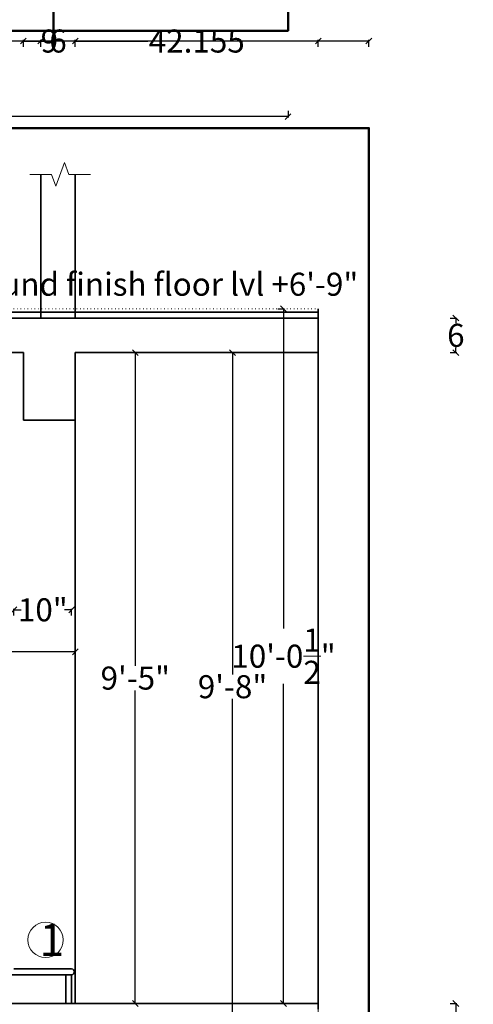
# Model space of a CAD drawing. Units: inches. Extents: x -60 to 284, y -245 to 257.
# Tile 5 of 10: x 193 to 272, y -159 to 12. Entities that reach past the tile are written whole.
import ezdxf

# ---------------------------------------------------------------- set-up
doc = ezdxf.new("R2010")
doc.units = ezdxf.units.IN
doc.header["$LTSCALE"] = 0.8
doc.header["$MEASUREMENT"] = 0
doc.linetypes.add('DOT', pattern=[6.35, 0, -6.35])
for name, color, linetype, lineweight in [('A-ANNO-DIMS', 2, 'Continuous', 18), ('A-ANNO-SYMB', 3, 'Continuous', 18), ('A-ANNO-TEXT', 3, 'Continuous', 18), ('A-ANNO-TTLB', 7, 'Continuous', 50), ('A-SECT', 7, 'Continuous', 35), ('A-SECT-OVHD', 8, 'DOT', 18), ('A-WALL', 7, 'Continuous', 50)]:
    doc.layers.add(name, color=color, linetype=linetype, lineweight=lineweight)
doc.styles.get("Standard").update_dxf_attribs({"font": 'arial.ttf'})
doc.dimstyles.get("Standard").update_dxf_attribs({"dimtxt": 4, "dimasz": 1, "dimexe": 0.18, "dimexo": 0.0625, "dimgap": 0.09, "dimtad": 0, "dimtih": 1, "dimtoh": 1, "dimzin": 0, "dimdsep": 46, "dimlunit": 4, "dimtxsty": 'Standard', "dimblk": 'OBLIQUE', "dimcen": 0.09, "dimadec": 0, "dimazin": 0, "dimtfac": 1, "dimtofl": 0, "dimtmove": 0, "dimatfit": 3, "dimfxl": 1, "dimfxlon": 1, "dimtolj": 1, "dimtzin": 0, "dimarcsym": 0})

# ---------------------------------------------------------------- blocks, each defined once
blk = doc.blocks.new('_Oblique')
at = {"color": 0, "linetype": 'ByBlock', "lineweight": -2}
blk.add_line((-0.5, -0.5), (0.5, 0.5), dxfattribs=at)
blk = doc.blocks.new('*D41')
at = {"layer": 'A-ANNO-DIMS', "color": 0, "lineweight": -2, "ltscale": 0.8, "transparency": 16777216}
for p, q in [((192.1, -91.86), (192.1, -90.68)), ((192.1, -90.86), (193.35, -90.86)), ((202.1, -90.86), (200.85, -90.86)), ((202.1, -91.86), (202.1, -90.68))]:
    blk.add_line(p, q, dxfattribs=at)
at = {"layer": 'Defpoints', "color": 0, "ltscale": 0.8, "transparency": 16777216}
for p in [(192.1, -90.86), (192.1, -168.75), (202.1, -168.75)]:
    blk.add_point(p, dxfattribs=at)
at = {"layer": 'A-ANNO-DIMS', "color": 0, "lineweight": -2, "ltscale": 0.8, "transparency": 16777216, "rotation": 180}
blk.add_blockref('_Oblique', (192.1, -90.86), dxfattribs=at)
at = {"layer": 'A-ANNO-DIMS', "color": 0, "lineweight": -2, "ltscale": 0.8, "transparency": 16777216}
blk.add_blockref('_Oblique', (202.1, -90.86), dxfattribs=at)
at = {"layer": 'A-ANNO-DIMS', "color": 0, "ltscale": 0.8, "transparency": 16777216, "insert": (197.1, -90.86), "char_height": 4, "attachment_point": 5}
blk.add_mtext('\\A1;10"', dxfattribs=at)
blk = doc.blocks.new('*D68')
at = {"layer": 'A-ANNO-DIMS', "color": 0, "lineweight": -2, "ltscale": 0.8, "transparency": 16777216}
for p, q in [((67.01, -97.15), (67.01, -98.33)), ((202.74, -97.15), (202.74, -98.33)), ((67.01, -98.15), (126.59, -98.15)), ((202.74, -98.15), (143.17, -98.15))]:
    blk.add_line(p, q, dxfattribs=at)
at = {"layer": 'Defpoints', "color": 0, "ltscale": 0.8, "transparency": 16777216}
for p in [(67.01, -93.21), (202.74, -93.21), (202.74, -98.15)]:
    blk.add_point(p, dxfattribs=at)
at = {"layer": 'A-ANNO-DIMS', "color": 0, "lineweight": -2, "ltscale": 0.8, "transparency": 16777216, "rotation": 180}
blk.add_blockref('_Oblique', (67.01, -98.15), dxfattribs=at)
at = {"layer": 'A-ANNO-DIMS', "color": 0, "lineweight": -2, "ltscale": 0.8, "transparency": 16777216}
blk.add_blockref('_Oblique', (202.74, -98.15), dxfattribs=at)
at = {"layer": 'A-ANNO-DIMS', "color": 0, "ltscale": 0.8, "transparency": 16777216, "insert": (134.88, -98.15), "char_height": 4, "attachment_point": 5}
blk.add_mtext('\\A1;11\'-3{\\H1x;\\S3/4;}"', dxfattribs=at)
blk = doc.blocks.new('*D69')
at = {"layer": 'A-ANNO-DIMS', "color": 0, "lineweight": -2, "ltscale": 0.8, "transparency": 16777216}
for p, q in [((212.15, -46.21), (213.33, -46.21)), ((213.15, -46.21), (213.15, -100.58)), ((213.15, -159.21), (213.15, -104.84)), ((212.15, -159.21), (213.33, -159.21))]:
    blk.add_line(p, q, dxfattribs=at)
at = {"layer": 'Defpoints', "color": 0, "ltscale": 0.8, "transparency": 16777216}
for p in [(212.05, -46.21), (213.15, -46.21), (212.05, -159.21)]:
    blk.add_point(p, dxfattribs=at)
at = {"layer": 'A-ANNO-DIMS', "color": 0, "lineweight": -2, "ltscale": 0.8, "transparency": 16777216}
for p, rotation in [((213.15, -46.21), 90), ((213.15, -159.21), 270)]:
    blk.add_blockref('_Oblique', p, dxfattribs=dict(at, rotation=rotation))
at = {"layer": 'A-ANNO-DIMS', "color": 0, "ltscale": 0.8, "transparency": 16777216, "insert": (213.15, -102.71), "char_height": 4, "attachment_point": 5}
blk.add_mtext('\\A1;9\'-5"', dxfattribs=at)
blk = doc.blocks.new('*D70')
at = {"layer": 'A-ANNO-DIMS', "color": 0, "lineweight": -2, "ltscale": 0.8, "transparency": 16777216}
for p, q in [((229.03, -46.21), (230.21, -46.21)), ((230.03, -46.21), (230.03, -102.08)), ((230.03, -162.21), (230.03, -106.34)), ((229.03, -162.21), (230.21, -162.21))]:
    blk.add_line(p, q, dxfattribs=at)
at = {"layer": 'Defpoints', "color": 0, "ltscale": 0.8, "transparency": 16777216}
for p in [(227.81, -46.21), (230.03, -46.21), (219.24, -162.21)]:
    blk.add_point(p, dxfattribs=at)
at = {"layer": 'A-ANNO-DIMS', "color": 0, "lineweight": -2, "ltscale": 0.8, "transparency": 16777216}
for p, rotation in [((230.03, -46.21), 90), ((230.03, -162.21), 270)]:
    blk.add_blockref('_Oblique', p, dxfattribs=dict(at, rotation=rotation))
at = {"layer": 'A-ANNO-DIMS', "color": 0, "ltscale": 0.8, "transparency": 16777216, "insert": (230.03, -104.21), "char_height": 4, "attachment_point": 5}
blk.add_mtext('\\A1;9\'-8"', dxfattribs=at)
blk = doc.blocks.new('*D71')
at = {"layer": 'A-ANNO-DIMS', "color": 0, "lineweight": -2, "ltscale": 0.8, "transparency": 16777216}
for p, q in [((237.88, -38.61), (239.06, -38.61)), ((238.88, -38.61), (238.88, -94.1)), ((238.88, -159.21), (238.88, -103.72)), ((237.88, -159.21), (239.06, -159.21))]:
    blk.add_line(p, q, dxfattribs=at)
at = {"layer": 'Defpoints', "color": 0, "ltscale": 0.8, "transparency": 16777216}
for p in [(235.46, -38.61), (238.88, -38.61), (235.46, -159.21)]:
    blk.add_point(p, dxfattribs=at)
at = {"layer": 'A-ANNO-DIMS', "color": 0, "lineweight": -2, "ltscale": 0.8, "transparency": 16777216}
for p, rotation in [((238.88, -38.61), 90), ((238.88, -159.21), 270)]:
    blk.add_blockref('_Oblique', p, dxfattribs=dict(at, rotation=rotation))
at = {"layer": 'A-ANNO-DIMS', "color": 0, "ltscale": 0.8, "transparency": 16777216, "insert": (238.88, -98.91), "char_height": 4, "attachment_point": 5}
blk.add_mtext('\\A1;10\'-0{\\H1x;\\S1/2;}"', dxfattribs=at)
blk = doc.blocks.new('*D89')
at = {"layer": 'A-ANNO-DIMS', "color": 0, "lineweight": -2, "ltscale": 0.8, "transparency": 16777216}
for p, q in [((0.09, -4.23), (0.09, -5.41)), ((239.66, -4.23), (239.66, -5.41)), ((0.09, -5.23), (113, -5.23)), ((239.66, -5.23), (126.75, -5.23))]:
    blk.add_line(p, q, dxfattribs=at)
at = {"layer": 'Defpoints', "color": 0, "ltscale": 0.8, "transparency": 16777216}
for p in [(0.09, 9.67), (239.66, 9.67), (239.66, -5.23)]:
    blk.add_point(p, dxfattribs=at)
at = {"layer": 'A-ANNO-DIMS', "color": 0, "lineweight": -2, "ltscale": 0.8, "transparency": 16777216, "rotation": 180}
blk.add_blockref('_Oblique', (0.09, -5.23), dxfattribs=at)
at = {"layer": 'A-ANNO-DIMS', "color": 0, "lineweight": -2, "ltscale": 0.8, "transparency": 16777216}
blk.add_blockref('_Oblique', (239.66, -5.23), dxfattribs=at)
at = {"layer": 'A-ANNO-DIMS', "color": 0, "ltscale": 0.8, "transparency": 16777216, "insert": (119.88, -5.23), "char_height": 4, "attachment_point": 5}
blk.add_mtext('\\A1;239.6', dxfattribs=at)
blk = doc.blocks.new('*D105')
at = {"layer": 'A-ANNO-DIMS', "color": 0, "lineweight": -2, "ltscale": 0.8, "transparency": 16777216}
for p, q in [((67.01, -241.38), (67.01, -242.56)), ((67.01, -242.38), (149.3, -242.38)), ((244.9, -242.38), (162.61, -242.38)), ((244.9, -241.38), (244.9, -242.56))]:
    blk.add_line(p, q, dxfattribs=at)
at = {"layer": 'Defpoints', "color": 0, "ltscale": 0.8, "transparency": 16777216}
for p in [(67.01, -159.21), (244.9, -171.21), (244.9, -242.38)]:
    blk.add_point(p, dxfattribs=at)
at = {"layer": 'A-ANNO-DIMS', "color": 0, "lineweight": -2, "ltscale": 0.8, "transparency": 16777216, "rotation": 180}
blk.add_blockref('_Oblique', (67.01, -242.38), dxfattribs=at)
at = {"layer": 'A-ANNO-DIMS', "color": 0, "lineweight": -2, "ltscale": 0.8, "transparency": 16777216}
blk.add_blockref('_Oblique', (244.9, -242.38), dxfattribs=at)
at = {"layer": 'A-ANNO-DIMS', "color": 0, "ltscale": 0.8, "transparency": 16777216, "insert": (155.96, -242.38), "char_height": 4, "attachment_point": 5}
blk.add_mtext('\\A1;177.9', dxfattribs=at)
blk = doc.blocks.new('*D107')
at = {"layer": 'A-ANNO-DIMS', "color": 0, "lineweight": -2, "ltscale": 0.8, "transparency": 16777216}
for p, q in [((267.79, -40.21), (268.97, -40.21)), ((268.79, -40.21), (268.79, -41.08)), ((268.79, -46.21), (268.79, -45.34)), ((267.79, -46.21), (268.97, -46.21))]:
    blk.add_line(p, q, dxfattribs=at)
at = {"layer": 'Defpoints', "color": 0, "ltscale": 0.8, "transparency": 16777216}
for p in [(244.9, -40.21), (244.9, -46.21), (268.79, -46.21)]:
    blk.add_point(p, dxfattribs=at)
at = {"layer": 'A-ANNO-DIMS', "color": 0, "lineweight": -2, "ltscale": 0.8, "transparency": 16777216}
for p, rotation in [((268.79, -40.21), 90), ((268.79, -46.21), 270)]:
    blk.add_blockref('_Oblique', p, dxfattribs=dict(at, rotation=rotation))
at = {"layer": 'A-ANNO-DIMS', "color": 0, "ltscale": 0.8, "transparency": 16777216, "insert": (268.79, -43.21), "char_height": 4, "attachment_point": 5}
blk.add_mtext('\\A1;6', dxfattribs=at)
blk = doc.blocks.new('*D108')
at = {"layer": 'A-ANNO-DIMS', "color": 0, "lineweight": -2, "ltscale": 0.8, "transparency": 16777216}
for p, q in [((267.79, -159.21), (268.97, -159.21)), ((268.79, -159.21), (268.79, -163.11)), ((268.79, -171.21), (268.79, -167.31)), ((267.79, -171.21), (268.97, -171.21))]:
    blk.add_line(p, q, dxfattribs=at)
at = {"layer": 'Defpoints', "color": 0, "ltscale": 0.8, "transparency": 16777216}
for p in [(244.9, -159.21), (244.9, -171.21), (268.79, -171.21)]:
    blk.add_point(p, dxfattribs=at)
at = {"layer": 'A-ANNO-DIMS', "color": 0, "lineweight": -2, "ltscale": 0.8, "transparency": 16777216}
for p, rotation in [((268.79, -159.21), 90), ((268.79, -171.21), 270)]:
    blk.add_blockref('_Oblique', p, dxfattribs=dict(at, rotation=rotation))
at = {"layer": 'A-ANNO-DIMS', "color": 0, "ltscale": 0.8, "transparency": 16777216, "insert": (268.79, -165.21), "char_height": 4, "attachment_point": 5}
blk.add_mtext('\\A1;12', dxfattribs=at)
blk = doc.blocks.new('*D109')
at = {"layer": 'A-ANNO-DIMS', "color": 0, "lineweight": -2, "ltscale": 0.8, "transparency": 16777216}
for p, q in [((196.74, 6.88), (196.74, 8.06)), ((196.74, 7.88), (198.33, 7.88)), ((202.74, 7.88), (201.15, 7.88)), ((202.74, 6.88), (202.74, 8.06))]:
    blk.add_line(p, q, dxfattribs=at)
at = {"layer": 'Defpoints', "color": 0, "ltscale": 0.8, "transparency": 16777216}
for p in [(202.74, 7.88), (196.74, -15.28), (202.74, -15.28)]:
    blk.add_point(p, dxfattribs=at)
at = {"layer": 'A-ANNO-DIMS', "color": 0, "lineweight": -2, "ltscale": 0.8, "transparency": 16777216, "rotation": 180}
blk.add_blockref('_Oblique', (196.74, 7.88), dxfattribs=at)
at = {"layer": 'A-ANNO-DIMS', "color": 0, "lineweight": -2, "ltscale": 0.8, "transparency": 16777216}
blk.add_blockref('_Oblique', (202.74, 7.88), dxfattribs=at)
at = {"layer": 'A-ANNO-DIMS', "color": 0, "ltscale": 0.8, "transparency": 16777216, "insert": (199.74, 7.88), "char_height": 4, "attachment_point": 5}
blk.add_mtext('\\A1;6', dxfattribs=at)
blk = doc.blocks.new('*D110')
at = {"layer": 'A-ANNO-DIMS', "color": 0, "lineweight": -2, "ltscale": 0.8, "transparency": 16777216}
for p, q in [((193.74, 6.88), (193.74, 8.06)), ((193.74, 7.88), (196.84, 7.88)), ((202.74, 7.88), (199.65, 7.88)), ((202.74, 6.88), (202.74, 8.06))]:
    blk.add_line(p, q, dxfattribs=at)
at = {"layer": 'Defpoints', "color": 0, "ltscale": 0.8, "transparency": 16777216}
for p in [(202.74, 7.88), (193.74, -57.93), (202.74, -57.93)]:
    blk.add_point(p, dxfattribs=at)
at = {"layer": 'A-ANNO-DIMS', "color": 0, "lineweight": -2, "ltscale": 0.8, "transparency": 16777216, "rotation": 180}
blk.add_blockref('_Oblique', (193.74, 7.88), dxfattribs=at)
at = {"layer": 'A-ANNO-DIMS', "color": 0, "lineweight": -2, "ltscale": 0.8, "transparency": 16777216}
blk.add_blockref('_Oblique', (202.74, 7.88), dxfattribs=at)
at = {"layer": 'A-ANNO-DIMS', "color": 0, "ltscale": 0.8, "transparency": 16777216, "insert": (198.24, 7.88), "char_height": 4, "attachment_point": 5}
blk.add_mtext('\\A1;9', dxfattribs=at)
blk = doc.blocks.new('*D111')
at = {"layer": 'A-ANNO-DIMS', "color": 0, "lineweight": -2, "ltscale": 0.8, "transparency": 16777216}
for p, q in [((-50.85, -46.21), (-52.03, -46.21)), ((-51.85, -46.21), (-51.85, -49.97)), ((-51.85, -57.93), (-51.85, -54.17)), ((-50.85, -57.93), (-52.03, -57.93))]:
    blk.add_line(p, q, dxfattribs=at)
at = {"layer": 'Defpoints', "color": 0, "ltscale": 0.8, "transparency": 16777216}
for p in [(193.74, -46.21), (-51.85, -57.93), (193.74, -57.93)]:
    blk.add_point(p, dxfattribs=at)
at = {"layer": 'A-ANNO-DIMS', "color": 0, "lineweight": -2, "ltscale": 0.8, "transparency": 16777216}
for p, rotation in [((-51.85, -46.21), 90), ((-51.85, -57.93), 270)]:
    blk.add_blockref('_Oblique', p, dxfattribs=dict(at, rotation=rotation))
at = {"layer": 'A-ANNO-DIMS', "color": 0, "ltscale": 0.8, "transparency": 16777216, "insert": (-51.85, -52.07), "char_height": 4, "attachment_point": 5}
blk.add_mtext('\\A1;11.717', dxfattribs=at)
blk = doc.blocks.new('*D112')
at = {"layer": 'A-ANNO-DIMS', "color": 0, "lineweight": -2, "ltscale": 0.8, "transparency": 16777216}
for p, q in [((202.74, 6.88), (202.74, 8.06)), ((202.74, 7.88), (215.33, 7.88)), ((244.9, 7.88), (232.31, 7.88)), ((244.9, 6.88), (244.9, 8.06))]:
    blk.add_line(p, q, dxfattribs=at)
at = {"layer": 'Defpoints', "color": 0, "ltscale": 0.8, "transparency": 16777216}
for p in [(244.9, 7.88), (202.74, -46.21), (244.9, -46.21)]:
    blk.add_point(p, dxfattribs=at)
at = {"layer": 'A-ANNO-DIMS', "color": 0, "lineweight": -2, "ltscale": 0.8, "transparency": 16777216, "rotation": 180}
blk.add_blockref('_Oblique', (202.74, 7.88), dxfattribs=at)
at = {"layer": 'A-ANNO-DIMS', "color": 0, "lineweight": -2, "ltscale": 0.8, "transparency": 16777216}
blk.add_blockref('_Oblique', (244.9, 7.88), dxfattribs=at)
at = {"layer": 'A-ANNO-DIMS', "color": 0, "ltscale": 0.8, "transparency": 16777216, "insert": (223.82, 7.88), "char_height": 4, "attachment_point": 5}
blk.add_mtext('\\A1;42.155', dxfattribs=at)
blk = doc.blocks.new('*D114')
at = {"layer": 'A-ANNO-DIMS', "color": 0, "lineweight": -2, "ltscale": 0.8, "transparency": 16777216}
for p, q in [((-36.75, 6.88), (-36.75, 8.06)), ((-36.75, 7.88), (100.05, 7.88)), ((253.69, 7.88), (116.89, 7.88)), ((253.69, 6.88), (253.69, 8.06))]:
    blk.add_line(p, q, dxfattribs=at)
at = {"layer": 'Defpoints', "color": 0, "ltscale": 0.8, "transparency": 16777216}
for p in [(253.69, 7.88), (-36.75, -7.22), (253.69, -7.22)]:
    blk.add_point(p, dxfattribs=at)
at = {"layer": 'A-ANNO-DIMS', "color": 0, "lineweight": -2, "ltscale": 0.8, "transparency": 16777216, "rotation": 180}
blk.add_blockref('_Oblique', (-36.75, 7.88), dxfattribs=at)
at = {"layer": 'A-ANNO-DIMS', "color": 0, "lineweight": -2, "ltscale": 0.8, "transparency": 16777216}
blk.add_blockref('_Oblique', (253.69, 7.88), dxfattribs=at)
at = {"layer": 'A-ANNO-DIMS', "color": 0, "ltscale": 0.8, "transparency": 16777216, "insert": (108.47, 7.88), "char_height": 4, "attachment_point": 5}
blk.add_mtext('\\A1;290.44', dxfattribs=at)

msp = doc.modelspace()

# ---------------------------------------------------------------- linework, layer by layer
at = {"layer": 'A-ANNO-SYMB', "ltscale": 0.8}
for points in [[(205.3572, -15.2818), (201.6094, -15.2818), (200.8594, -13.2212), (199.3594, -17.3424), (198.6094, -15.2818), (194.8616, -15.2818)], [(244.8977, -159.0289), (244.8977, -162.6103), (242.8371, -163.3603), (246.9583, -164.8603), (244.8977, -165.6103), (244.8977, -173.978)]]:
    msp.add_lwpolyline(points, dxfattribs=at)
msp.add_circle((197.5773, -148.1613), 3.069, dxfattribs=at)
at = {"layer": 'A-ANNO-TTLB', "ltscale": 0.8}
for points in [[(0.0867, 122.666), (239.6639, 122.666), (239.6639, 9.666), (0.0867, 9.666)], [(-36.7489, -7.223), (253.6882, -7.223), (253.6882, -227.2835), (-36.7489, -227.2835)]]:
    msp.add_lwpolyline(points, close=True, dxfattribs=at)
at = {"layer": 'A-SECT', "ltscale": 0.8}
for p, q in [((196.7426, -40.2089), (196.7426, -15.2818)), ((202.7426, -15.2818), (202.7426, -40.2089)), ((244.8977, -159.2089), (244.8977, -38.6089)), ((161.0139, -40.2089), (244.8977, -40.2089)), ((202.7426, -40.2089), (196.7426, -40.2089)), ((193.7426, -46.2089), (187.7426, -46.2089)), ((193.7426, -57.9262), (193.7426, -46.2089)), ((202.7426, -46.2089), (202.7426, -159.2089)), ((202.7426, -46.2089), (244.8977, -46.2089)), ((202.7426, -57.9262), (193.7426, -57.9262)), ((202.1002, -153.2089), (192.1002, -153.2089)), ((202.1002, -154.2089), (191.1002, -154.2089)), ((201.1002, -159.2089), (201.1002, -154.2089)), ((202.1002, -159.2089), (202.1002, -154.2089)), ((244.8977, -159.2089), (82.0139, -159.2089)), ((244.8977, -159.2089), (244.8977, -160.2089))]:
    msp.add_line(p, q, dxfattribs=at)
msp.add_lwpolyline([(161.0139, -39.2089), (244.8977, -39.2089)], dxfattribs=at)
msp.add_arc((202.1002, -153.7089), 0.5, 270, 90, dxfattribs=at)
at = {"layer": 'A-SECT-OVHD', "ltscale": 0.1}
msp.add_lwpolyline([(161.0139, -38.6089), (244.8977, -38.6089)], dxfattribs=at)
at = {"layer": 'A-WALL'}
msp.add_lwpolyline([(198.9361, 9.666), (198.9361, 21.666), (159.9361, 21.666), (79.9361, 21.666), (37.9361, 21.666), (27.9361, 21.666), (27.9361, 9.666)], dxfattribs=at)

# ---------------------------------------------------------------- texts
at = {"layer": 'A-ANNO-TEXT', "ltscale": 0.8, "attachment_point": 1}
for s, width, gutter_width, insert, char_height in [('ground finish floor lvl +6\'-9"', 97.551324, 1, (181.3842, -32.3395), 4), ('1', 28.020867, 2.8021, (196.5451, -145.3478), 5.6042)]:
    msp.add_mtext_dynamic_manual_height_columns(s, width=width, gutter_width=gutter_width, heights=[0], dxfattribs=dict(at, insert=insert, char_height=char_height))

# ---------------------------------------------------------------- dimensions: what is measured, and where the dimension line sits
at = {"layer": 'A-ANNO-DIMS', "ltscale": 0.8}
for base, p1, p2, override, picture, middle in [((253.6882, 7.877), (-36.7489, -7.223), (253.6882, -7.223), {"dimdec": 2, "dimlfac": 1, "dimrnd": 0, "dimzin": 0, "dimdsep": 46, "dimlunit": 2}, '*D114', (108.4697, 7.877)), ((202.7426, 7.877), (193.7426, -57.9262), (202.7426, -57.9262), {"dimdec": 0, "dimlfac": 1, "dimrnd": 0, "dimzin": 0, "dimdsep": 46, "dimlunit": 2}, '*D110', (198.2426, 7.877)), ((202.7426, 7.877), (196.7426, -15.2818), (202.7426, -15.2818), {"dimdec": 0, "dimlfac": 1, "dimrnd": 0, "dimzin": 0, "dimdsep": 46, "dimlunit": 2}, '*D109', (199.7426, 7.877)), ((244.8977, 7.877), (202.7426, -46.2089), (244.8977, -46.2089), {"dimdec": 3, "dimlfac": 1, "dimrnd": 0, "dimzin": 0, "dimdsep": 46, "dimlunit": 2}, '*D112', (223.8201, 7.877)), ((239.6639, -5.234), (0.0867, 9.666), (239.6639, 9.666), {"dimdec": 1, "dimlfac": 1, "dimrnd": 0, "dimzin": 0, "dimdsep": 46, "dimlunit": 2}, '*D89', (119.8753, -5.234)), ((192.1002, -90.8616), (202.1002, -168.7549), (192.1002, -168.7549), {"dimclrd": 0, "dimclre": 0, "dimclrt": 0}, '*D41', (197.1002, -90.8616)), ((202.7426, -98.1513), (67.0139, -93.2089), (202.7426, -93.2089), {"dimclrd": 0, "dimclre": 0, "dimclrt": 0}, '*D68', (134.8782, -98.1513)), ((244.8977, -242.3835), (67.0139, -159.2089), (244.8977, -171.2089), {"dimdec": 1, "dimlfac": 1, "dimrnd": 0, "dimzin": 0, "dimdsep": 46, "dimlunit": 2}, '*D105', (155.9558, -242.3835))]:
    dim = msp.add_linear_dim(base=base, p1=p1, p2=p2, dimstyle='Standard', override=override, dxfattribs=at)
    dim.commit()
    dim.dimension.update_dxf_attribs({"geometry": picture, "text_midpoint": middle})
for base, p1, p2, override, picture, middle in [((238.8784, -38.6089), (235.4628, -159.2089), (235.4628, -38.6089), {"dimclrd": 0, "dimclre": 0, "dimclrt": 0}, '*D71', (238.8784, -98.9089)), ((268.7882, -46.2089), (244.8977, -40.2089), (244.8977, -46.2089), {"dimdec": 0, "dimlfac": 1, "dimrnd": 0, "dimzin": 0, "dimdsep": 46, "dimlunit": 2}, '*D107', (268.7882, -43.2089)), ((-51.8489, -57.9262), (193.7426, -46.2089), (193.7426, -57.9262), {"dimdec": 3, "dimlfac": 1, "dimrnd": 0, "dimzin": 0, "dimdsep": 46, "dimlunit": 2}, '*D111', (-51.8489, -52.0675)), ((213.1492, -46.2089), (212.0462, -159.2089), (212.0462, -46.2089), {"dimclrd": 0, "dimclre": 0, "dimclrt": 0}, '*D69', (213.1492, -102.7089)), ((230.0275, -46.2089), (219.2361, -162.2089), (227.8081, -46.2089), {"dimclrd": 0, "dimclre": 0, "dimclrt": 0}, '*D70', (230.0275, -104.2089)), ((268.7882, -171.2089), (244.8977, -159.2089), (244.8977, -171.2089), {"dimdec": 0, "dimlfac": 1, "dimrnd": 0, "dimzin": 0, "dimdsep": 46, "dimlunit": 2}, '*D108', (268.7882, -165.2089))]:
    dim = msp.add_linear_dim(base=base, p1=p1, p2=p2, angle=90, dimstyle='Standard', override=override, dxfattribs=at)
    dim.commit()
    dim.dimension.update_dxf_attribs({"geometry": picture, "text_midpoint": middle})

doc.saveas('drawing.dxf')
